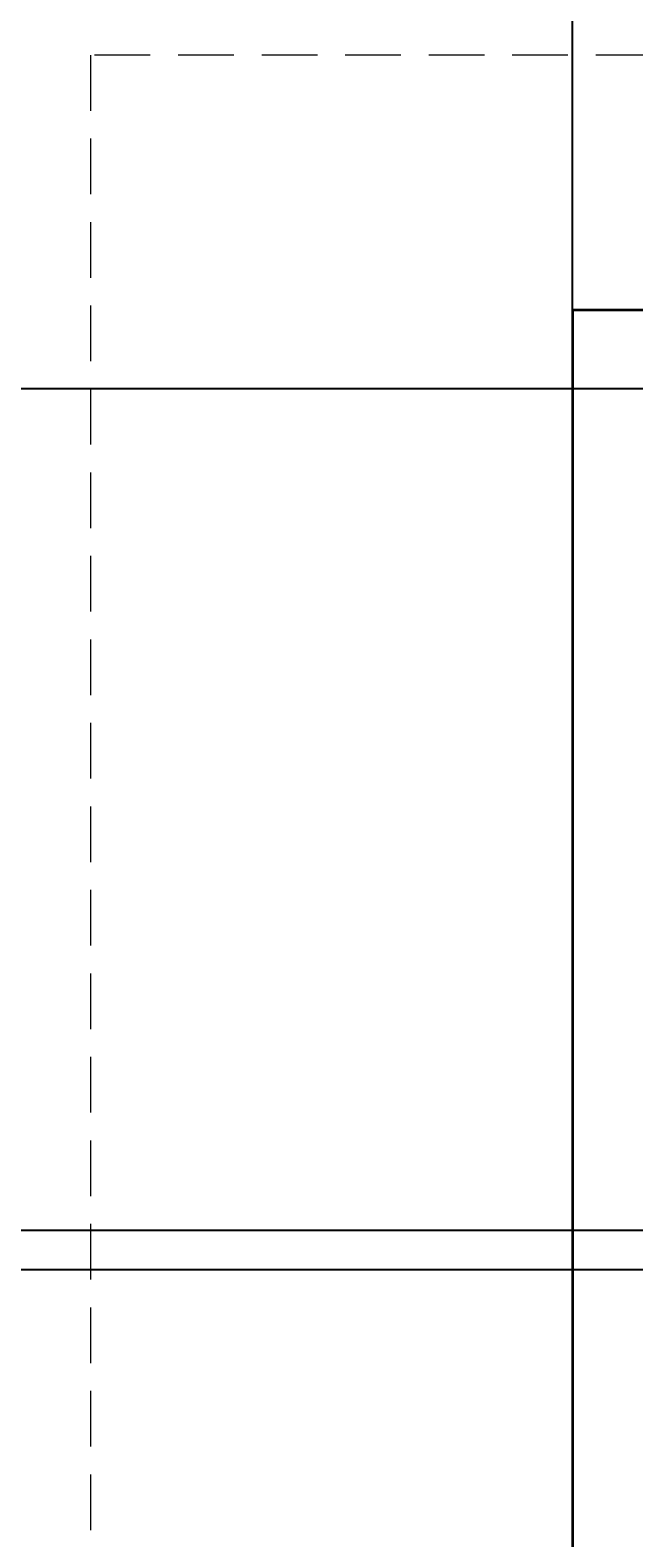
# Model space of a CAD drawing. Units: inches. Extents: x 1770 to 2988, y 1161 to 3221.
# Tile 12 of 44: x 2090 to 2159, y 2237 to 2409. Entities that reach past the tile are written whole.
import ezdxf

# ---------------------------------------------------------------- set-up
doc = ezdxf.new("R2010")
doc.units = ezdxf.units.IN
doc.linetypes.add('DASHED2', pattern=[9.525, 6.35, -3.175])
for name, color, linetype, lineweight in [('A-ANNO-DIMS', 2, 'Continuous', 18), ('A-ROOF-OVHD', 7, 'DASHED2', 18), ('A-WALL', 7, 'Continuous', 35)]:
    doc.layers.add(name, color=color, linetype=linetype, lineweight=lineweight)
doc.styles.get("Standard").update_dxf_attribs({"font": 'arial.ttf'})
doc.dimstyles.get("Standard").update_dxf_attribs({"dimtxt": 0.18, "dimasz": 0.18, "dimexe": 0.18, "dimexo": 0.0625, "dimgap": 0.09, "dimtad": 0, "dimtih": 1, "dimtoh": 1, "dimdec": 4, "dimzin": 0, "dimdsep": 46, "dimtxsty": 'Standard', "dimcen": 0.09, "dimadec": 0, "dimazin": 0, "dimtfac": 1, "dimtdec": 4, "dimtofl": 0, "dimtmove": 0, "dimatfit": 3, "dimfxl": 1, "dimtolj": 1, "dimtzin": 0, "dimarcsym": 0})

# ---------------------------------------------------------------- blocks, each defined once
blk = doc.blocks.new('*D64')
at = {"layer": 'A-ANNO-DIMS', "color": 0, "lineweight": -2, "transparency": 16777216}
for p, q in [((2151.7, 2376.76), (2151.7, 2570.7)), ((2151.88, 2570.52), (2179.09, 2570.52)), ((2207.1, 2570.52), (2179.88, 2570.52)), ((2207.28, 2376.76), (2207.28, 2570.7))]:
    blk.add_line(p, q, dxfattribs=at)
at = {"layer": 'A-ANNO-DIMS', "color": 0, "transparency": 16777216}
for points in [[(2151.88, 2570.55), (2151.88, 2570.49), (2151.7, 2570.52)], [(2207.1, 2570.55), (2207.1, 2570.49), (2207.28, 2570.52)]]:
    blk.add_solid(points, dxfattribs=at)
at = {"layer": 'Defpoints', "color": 0, "transparency": 16777216}
for p in [(2207.28, 2570.52), (2151.7, 2376.7), (2207.28, 2376.7)]:
    blk.add_point(p, dxfattribs=at)
at = {"layer": 'A-ANNO-DIMS', "color": 0, "transparency": 16777216, "insert": (2179.49, 2570.52), "char_height": 0.18, "attachment_point": 5}
blk.add_mtext('\\A1;55.58', dxfattribs=at)
blk = doc.blocks.new('*D72')
at = {"layer": 'A-ANNO-DIMS', "color": 0, "lineweight": -2, "transparency": 16777216}
for p, q in [((2456.13, 2267.2), (1907.1, 2267.2)), ((1907.28, 2267.02), (1907.28, 2221.63)), ((1907.28, 2175.88), (1907.28, 2221.27)), ((2456.13, 2175.7), (1907.1, 2175.7))]:
    blk.add_line(p, q, dxfattribs=at)
at = {"layer": 'A-ANNO-DIMS', "color": 0, "transparency": 16777216}
for points in [[(1907.25, 2267.02), (1907.31, 2267.02), (1907.28, 2267.2)], [(1907.25, 2175.88), (1907.31, 2175.88), (1907.28, 2175.7)]]:
    blk.add_solid(points, dxfattribs=at)
at = {"layer": 'Defpoints', "color": 0, "transparency": 16777216}
for p in [(1907.28, 2267.2), (2456.2, 2267.2), (2456.2, 2175.7)]:
    blk.add_point(p, dxfattribs=at)
at = {"layer": 'A-ANNO-DIMS', "color": 0, "transparency": 16777216, "insert": (1907.28, 2221.45), "char_height": 0.18, "attachment_point": 5}
blk.add_mtext('\\A1;91.5', dxfattribs=at)
blk = doc.blocks.new('*D73')
at = {"layer": 'A-ANNO-DIMS', "color": 0, "lineweight": -2, "transparency": 16777216}
for p, q in [((2456.13, 2367.7), (1907.1, 2367.7)), ((1907.28, 2367.52), (1907.28, 2319.88)), ((1907.28, 2271.88), (1907.28, 2319.52)), ((2456.13, 2271.7), (1907.1, 2271.7))]:
    blk.add_line(p, q, dxfattribs=at)
at = {"layer": 'A-ANNO-DIMS', "color": 0, "transparency": 16777216}
for points in [[(1907.25, 2367.52), (1907.31, 2367.52), (1907.28, 2367.7)], [(1907.25, 2271.88), (1907.31, 2271.88), (1907.28, 2271.7)]]:
    blk.add_solid(points, dxfattribs=at)
at = {"layer": 'Defpoints', "color": 0, "transparency": 16777216}
for p in [(1907.28, 2367.7), (2456.2, 2367.7), (2456.2, 2271.7)]:
    blk.add_point(p, dxfattribs=at)
at = {"layer": 'A-ANNO-DIMS', "color": 0, "transparency": 16777216, "insert": (1907.28, 2319.7), "char_height": 0.18, "attachment_point": 5}
blk.add_mtext('\\A1;96', dxfattribs=at)
blk = doc.blocks.new('*D79')
at = {"layer": 'A-ANNO-DIMS', "color": 0, "lineweight": -2, "transparency": 16777216}
for p, q in [((2151.7, 1610.26), (2151.7, 2570.7)), ((2151.88, 2570.52), (2177.78, 2570.52)), ((2204.48, 2570.52), (2178.57, 2570.52)), ((2204.66, 1610.26), (2204.66, 2570.7))]:
    blk.add_line(p, q, dxfattribs=at)
at = {"layer": 'A-ANNO-DIMS', "color": 0, "transparency": 16777216}
for points in [[(2151.88, 2570.55), (2151.88, 2570.49), (2151.7, 2570.52)], [(2204.48, 2570.55), (2204.48, 2570.49), (2204.66, 2570.52)]]:
    blk.add_solid(points, dxfattribs=at)
at = {"layer": 'Defpoints', "color": 0, "transparency": 16777216}
for p in [(2204.66, 2570.52), (2151.7, 1610.2), (2204.66, 1610.2)]:
    blk.add_point(p, dxfattribs=at)
at = {"layer": 'A-ANNO-DIMS', "color": 0, "transparency": 16777216, "insert": (2178.18, 2570.52), "char_height": 0.18, "attachment_point": 5}
blk.add_mtext('\\A1;52.96', dxfattribs=at)

msp = doc.modelspace()

# ---------------------------------------------------------------- linework, layer by layer
at = {"layer": 'A-ROOF-OVHD'}
for p, q in [((2656.0216, 2405.7876), (2096.7313, 2405.7876)), ((2096.7313, 2405.7876), (2096.7313, 1610.2021))]:
    msp.add_line(p, q, dxfattribs=at)
at = {"layer": 'A-WALL'}
for q in [(2151.696, 1610.2021), (2625.696, 2376.7021)]:
    msp.add_line((2151.696, 2376.7021), q, dxfattribs=at)

# ---------------------------------------------------------------- dimensions: what is measured, and where the dimension line sits
at = {"layer": 'A-ANNO-DIMS'}
for base, p1, p2, picture, middle in [((2207.2776, 2570.5247), (2151.696, 2376.7021), (2207.2776, 2376.7021), '*D64', (2179.4868, 2570.5247)), ((2204.6568, 2570.5247), (2151.696, 1610.2021), (2204.6568, 1610.2021), '*D79', (2178.1764, 2570.5247))]:
    dim = msp.add_linear_dim(base=base, p1=p1, p2=p2, dimstyle='Standard', override={"dimdec": 2, "dimlfac": 1, "dimrnd": 0, "dimzin": 0, "dimdsep": 46, "dimlunit": 2}, dxfattribs=at)
    dim.commit()
    dim.dimension.update_dxf_attribs({"geometry": picture, "text_midpoint": middle})
for base, p1, p2, override, picture, middle in [((1907.2844, 2367.7021), (2456.196, 2271.7021), (2456.196, 2367.7021), {"dimdec": 0, "dimlfac": 1, "dimrnd": 0, "dimzin": 0, "dimdsep": 46, "dimlunit": 2}, '*D73', (1907.2844, 2319.7021)), ((1907.2844, 2267.2021), (2456.196, 2175.7021), (2456.196, 2267.2021), {"dimdec": 1, "dimlfac": 1, "dimrnd": 0, "dimzin": 0, "dimdsep": 46, "dimlunit": 2}, '*D72', (1907.2844, 2221.4521))]:
    dim = msp.add_linear_dim(base=base, p1=p1, p2=p2, angle=90, dimstyle='Standard', override=override, dxfattribs=at)
    dim.commit()
    dim.dimension.update_dxf_attribs({"geometry": picture, "text_midpoint": middle})

doc.saveas('drawing.dxf')
